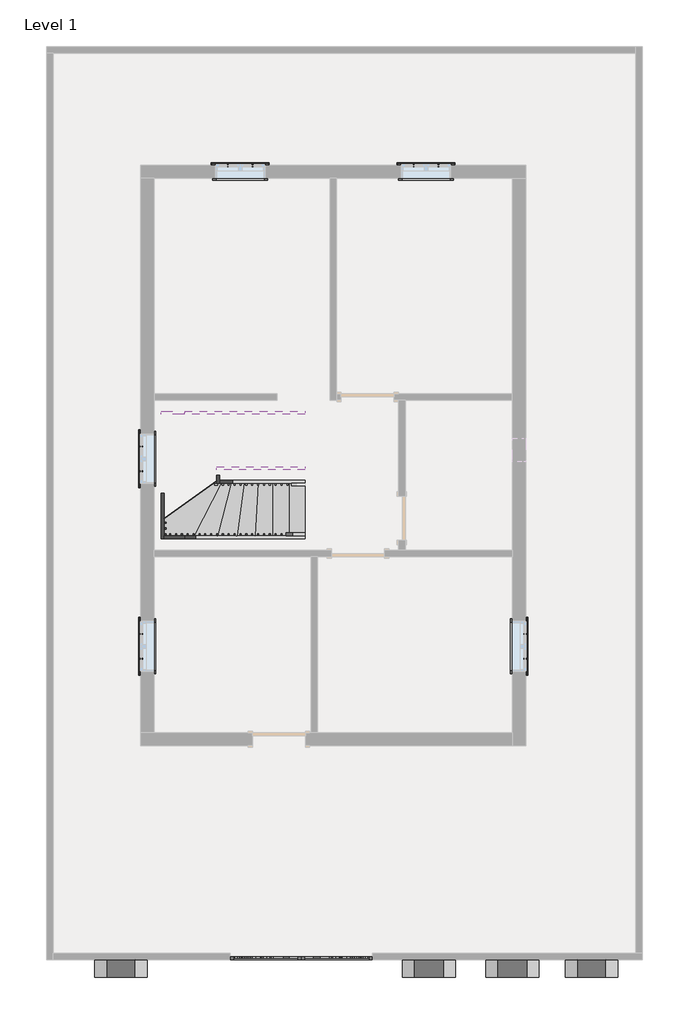
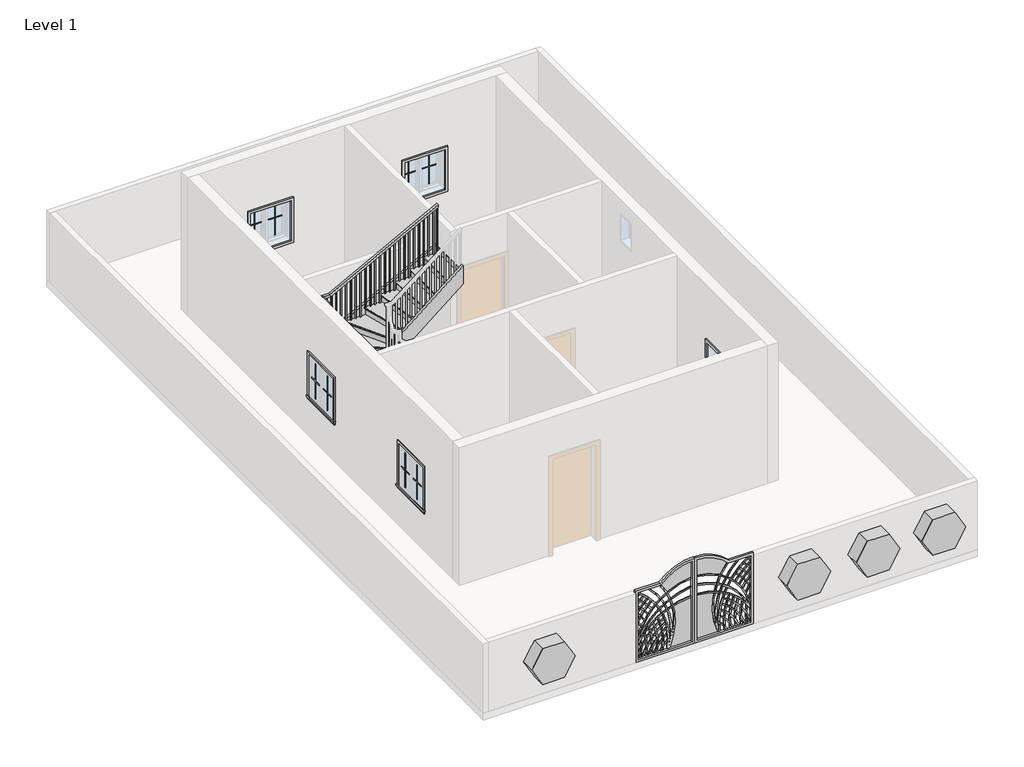
# One storey, part 2 of 2: 22 proxies, 8 members, 1 railing, 1 stair flight.
"""IFC4 building model written with IfcOpenShell, lengths in millimetres."""

from ifc_helpers import new_model, si_unit, frame, origin, place, context, project, spatial, polyline, outline, extrude, faceted_brep, transform, mapped, element, save
from components import generic_models_6bc30956, generic_models_2_generic_models_2_a86c904f, muntin_pattern_2x2_muntin_pattern_2x2_b3fe6957, muntin_pattern_2x2_muntin_pattern_2x2_3e0ecaf2, trim_window_exterior_flat_with_sill_41619996, trim_window_interior_flat_picture_frame_51c85655, stair_flight_5a9f065b

model = new_model("IFC4")

# Units and contexts
model_context = context("Model", 3, world=origin())
ifc_project = project(units=[si_unit("LENGTHUNIT", "METRE", prefix="MILLI")], contexts=[model_context])

# Site, building, storey
site = spatial("IfcSite", under=ifc_project)
building = spatial("IfcBuilding", under=site)
storey = spatial("IfcBuildingStorey", under=building, Name="Level 1", Elevation=0.0)

# Proxies
placement = place(None, origin())
generic_models_shape = generic_models_6bc30956(model_context)
element("IfcBuildingElementProxy", 1, Name="Generic Models", at=placement, inside=storey, context=model_context, shape_type="MappedRepresentation", body=[
    mapped(generic_models_shape, transform((-1831.5949167, -8550.141091, 0.0), x_axis=(1.0, 0.0, 0.0), y_axis=(0.0, 1.0, 0.0), z_axis=(0.0, 0.0, 1.0))),
])
generic_models_2_generic_models_2_shape = generic_models_2_generic_models_2_a86c904f(model_context)
element("IfcBuildingElementProxy", 2, Name="Generic Models 2 : Generic Models 2", ObjectType="Generic Models 2 : Generic Models 2", at=placement, inside=storey, context=model_context, shape_type="MappedRepresentation", body=[
    mapped(generic_models_2_generic_models_2_shape, transform((0.0, 0.0, 0.0), x_axis=(1.0, 0.0, 0.0), y_axis=(0.0, 1.0, 0.0), z_axis=(0.0, 0.0, 1.0))),
])
muntin_pattern_2x2_muntin_pattern_2x2_shape = muntin_pattern_2x2_muntin_pattern_2x2_b3fe6957(model_context)
element("IfcBuildingElementProxy", 3, Name="Muntin Pattern_2x2 : Muntin Pattern_2x2", ObjectType="Muntin Pattern_2x2 : Muntin Pattern_2x2", at=placement, inside=storey, context=model_context, shape_type="MappedRepresentation", body=[
    mapped(muntin_pattern_2x2_muntin_pattern_2x2_shape, transform((-3096.8324167, 5150.2179147, 984.25), x_axis=(1.0, 0.0, 0.0), y_axis=(0.0, 1.0, 0.0), z_axis=(0.0, 0.0, 1.0))),
])
element("IfcBuildingElementProxy", 4, Name="Muntin Pattern_2x2 : Muntin Pattern_2x2", ObjectType="Muntin Pattern_2x2 : Muntin Pattern_2x2", at=placement, inside=storey, context=model_context, shape_type="MappedRepresentation", body=[
    mapped(muntin_pattern_2x2_muntin_pattern_2x2_shape, transform((122.6175833, 5150.2179147, 984.25), x_axis=(1.0, 0.0, 0.0), y_axis=(0.0, 1.0, 0.0), z_axis=(0.0, 0.0, 1.0))),
])
element("IfcBuildingElementProxy", 5, Name="Muntin Pattern_2x2 : Muntin Pattern_2x2", ObjectType="Muntin Pattern_2x2 : Muntin Pattern_2x2", at=placement, inside=storey, context=model_context, shape_type="MappedRepresentation", body=[
    mapped(muntin_pattern_2x2_muntin_pattern_2x2_shape, transform((-4597.0199167, -3388.9445853, 984.25), x_axis=(0.0, 1.0, 0.0), y_axis=(-1.0, 0.0, 0.0), z_axis=(0.0, 0.0, 1.0))),
])
element("IfcBuildingElementProxy", 6, Name="Muntin Pattern_2x2 : Muntin Pattern_2x2", ObjectType="Muntin Pattern_2x2 : Muntin Pattern_2x2", at=placement, inside=storey, context=model_context, shape_type="MappedRepresentation", body=[
    mapped(muntin_pattern_2x2_muntin_pattern_2x2_shape, transform((2051.4300833, -2960.3195853, 984.25), x_axis=(0.0, -1.0, 0.0), y_axis=(1.0, 0.0, 0.0), z_axis=(0.0, 0.0, 1.0))),
])
element("IfcBuildingElementProxy", 7, Name="Muntin Pattern_2x2 : Muntin Pattern_2x2", ObjectType="Muntin Pattern_2x2 : Muntin Pattern_2x2", at=placement, inside=storey, context=model_context, shape_type="MappedRepresentation", body=[
    mapped(muntin_pattern_2x2_muntin_pattern_2x2_shape, transform((-4597.0199167, -140.9195853, 984.25), x_axis=(0.0, 1.0, 0.0), y_axis=(-1.0, 0.0, 0.0), z_axis=(0.0, 0.0, 1.0))),
])
muntin_pattern_2x2_muntin_pattern_2x2_2_shape = muntin_pattern_2x2_muntin_pattern_2x2_3e0ecaf2(model_context)
element("IfcBuildingElementProxy", 8, Name="Muntin Pattern_2x2 : Muntin Pattern_2x2", ObjectType="Muntin Pattern_2x2 : Muntin Pattern_2x2", at=placement, inside=storey, context=model_context, shape_type="MappedRepresentation", body=[
    mapped(muntin_pattern_2x2_muntin_pattern_2x2_2_shape, transform((-2668.2074167, 5150.2179147, 984.25), x_axis=(-1.0, 0.0, 0.0), y_axis=(0.0, -1.0, 0.0), z_axis=(0.0, 0.0, 1.0))),
])
element("IfcBuildingElementProxy", 9, Name="Muntin Pattern_2x2 : Muntin Pattern_2x2", ObjectType="Muntin Pattern_2x2 : Muntin Pattern_2x2", at=placement, inside=storey, context=model_context, shape_type="MappedRepresentation", body=[
    mapped(muntin_pattern_2x2_muntin_pattern_2x2_2_shape, transform((551.2425833, 5150.2179147, 984.25), x_axis=(-1.0, 0.0, 0.0), y_axis=(0.0, -1.0, 0.0), z_axis=(0.0, 0.0, 1.0))),
])
element("IfcBuildingElementProxy", 10, Name="Muntin Pattern_2x2 : Muntin Pattern_2x2", ObjectType="Muntin Pattern_2x2 : Muntin Pattern_2x2", at=placement, inside=storey, context=model_context, shape_type="MappedRepresentation", body=[
    mapped(muntin_pattern_2x2_muntin_pattern_2x2_2_shape, transform((-4597.0199167, -2960.3195853, 984.25), x_axis=(0.0, -1.0, 0.0), y_axis=(1.0, 0.0, 0.0), z_axis=(0.0, 0.0, 1.0))),
])
element("IfcBuildingElementProxy", 11, Name="Muntin Pattern_2x2 : Muntin Pattern_2x2", ObjectType="Muntin Pattern_2x2 : Muntin Pattern_2x2", at=placement, inside=storey, context=model_context, shape_type="MappedRepresentation", body=[
    mapped(muntin_pattern_2x2_muntin_pattern_2x2_2_shape, transform((2051.4300833, -3388.9445853, 984.25), x_axis=(0.0, 1.0, 0.0), y_axis=(-1.0, 0.0, 0.0), z_axis=(0.0, 0.0, 1.0))),
])
element("IfcBuildingElementProxy", 12, Name="Muntin Pattern_2x2 : Muntin Pattern_2x2", ObjectType="Muntin Pattern_2x2 : Muntin Pattern_2x2", at=placement, inside=storey, context=model_context, shape_type="MappedRepresentation", body=[
    mapped(muntin_pattern_2x2_muntin_pattern_2x2_2_shape, transform((-4597.0199167, 287.7054147, 984.25), x_axis=(0.0, -1.0, 0.0), y_axis=(1.0, 0.0, 0.0), z_axis=(0.0, 0.0, 1.0))),
])
trim_window_exterior_flat_with_sill_shape = trim_window_exterior_flat_with_sill_41619996(model_context)
element("IfcBuildingElementProxy", 13, Name="Trim-Window-Exterior-Flat : with Sill", ObjectType="Trim-Window-Exterior-Flat : with Sill", at=placement, inside=storey, context=model_context, shape_type="MappedRepresentation", body=[
    mapped(trim_window_exterior_flat_with_sill_shape, transform((-2882.5199167, 5159.7429147, 1828.8), x_axis=(-1.0, 0.0, 0.0), y_axis=(0.0, 0.0, 1.0), z_axis=(0.0, 1.0, 0.0))),
])
element("IfcBuildingElementProxy", 14, Name="Trim-Window-Exterior-Flat : with Sill", ObjectType="Trim-Window-Exterior-Flat : with Sill", at=placement, inside=storey, context=model_context, shape_type="MappedRepresentation", body=[
    mapped(trim_window_exterior_flat_with_sill_shape, transform((336.9300833, 5159.7429147, 1828.8), x_axis=(-1.0, 0.0, 0.0), y_axis=(0.0, 0.0, 1.0), z_axis=(0.0, 1.0, 0.0))),
])
element("IfcBuildingElementProxy", 15, Name="Trim-Window-Exterior-Flat : with Sill", ObjectType="Trim-Window-Exterior-Flat : with Sill", at=placement, inside=storey, context=model_context, shape_type="MappedRepresentation", body=[
    mapped(trim_window_exterior_flat_with_sill_shape, transform((-4606.5449167, -3174.6320853, 1828.8), x_axis=(0.0, -1.0, 0.0), y_axis=(0.0, 0.0, 1.0), z_axis=(-1.0, 0.0, 0.0))),
])
element("IfcBuildingElementProxy", 16, Name="Trim-Window-Exterior-Flat : with Sill", ObjectType="Trim-Window-Exterior-Flat : with Sill", at=placement, inside=storey, context=model_context, shape_type="MappedRepresentation", body=[
    mapped(trim_window_exterior_flat_with_sill_shape, transform((2060.9550833, -3174.6320853, 1828.8), x_axis=(0.0, 1.0, 0.0), y_axis=(0.0, 0.0, 1.0), z_axis=(1.0, 0.0, 0.0))),
])
element("IfcBuildingElementProxy", 17, Name="Trim-Window-Exterior-Flat : with Sill", ObjectType="Trim-Window-Exterior-Flat : with Sill", at=placement, inside=storey, context=model_context, shape_type="MappedRepresentation", body=[
    mapped(trim_window_exterior_flat_with_sill_shape, transform((-4606.5449167, 73.3929147, 1828.8), x_axis=(0.0, -1.0, 0.0), y_axis=(0.0, 0.0, 1.0), z_axis=(-1.0, 0.0, 0.0))),
])
trim_window_interior_flat_picture_frame_shape = trim_window_interior_flat_picture_frame_51c85655(model_context)
element("IfcBuildingElementProxy", 18, Name="Trim-Window-Interior-Flat : Picture Frame", ObjectType="Trim-Window-Interior-Flat : Picture Frame", at=placement, inside=storey, context=model_context, shape_type="MappedRepresentation", body=[
    mapped(trim_window_interior_flat_picture_frame_shape, transform((-2882.5199167, 4931.1429147, 1828.8), x_axis=(1.0, 0.0, 0.0), y_axis=(0.0, 0.0, 1.0), z_axis=(0.0, -1.0, 0.0))),
])
element("IfcBuildingElementProxy", 19, Name="Trim-Window-Interior-Flat : Picture Frame", ObjectType="Trim-Window-Interior-Flat : Picture Frame", at=placement, inside=storey, context=model_context, shape_type="MappedRepresentation", body=[
    mapped(trim_window_interior_flat_picture_frame_shape, transform((336.9300833, 4931.1429147, 1828.8), x_axis=(1.0, 0.0, 0.0), y_axis=(0.0, 0.0, 1.0), z_axis=(0.0, -1.0, 0.0))),
])
element("IfcBuildingElementProxy", 20, Name="Trim-Window-Interior-Flat : Picture Frame", ObjectType="Trim-Window-Interior-Flat : Picture Frame", at=placement, inside=storey, context=model_context, shape_type="MappedRepresentation", body=[
    mapped(trim_window_interior_flat_picture_frame_shape, transform((-4377.9449167, -3174.6320853, 1828.8), x_axis=(0.0, 1.0, 0.0), y_axis=(0.0, 0.0, 1.0), z_axis=(1.0, 0.0, 0.0))),
])
element("IfcBuildingElementProxy", 21, Name="Trim-Window-Interior-Flat : Picture Frame", ObjectType="Trim-Window-Interior-Flat : Picture Frame", at=placement, inside=storey, context=model_context, shape_type="MappedRepresentation", body=[
    mapped(trim_window_interior_flat_picture_frame_shape, transform((1832.3550833, -3174.6320853, 1828.8), x_axis=(0.0, -1.0, 0.0), y_axis=(0.0, 0.0, 1.0), z_axis=(-1.0, 0.0, 0.0))),
])
element("IfcBuildingElementProxy", 22, Name="Trim-Window-Interior-Flat : Picture Frame", ObjectType="Trim-Window-Interior-Flat : Picture Frame", at=placement, inside=storey, context=model_context, shape_type="MappedRepresentation", body=[
    mapped(trim_window_interior_flat_picture_frame_shape, transform((-4377.9449167, 73.3929147, 1828.8), x_axis=(0.0, 1.0, 0.0), y_axis=(0.0, 0.0, 1.0), z_axis=(1.0, 0.0, 0.0))),
])

# Members
element("IfcMember", 23, ObjectType="Stringer - 2\" Width", at=placement, inside=storey, context=model_context, shape_type="SweptSolid", body=[
    extrude(outline(polyline([(0.0, -1761.7449167), (229.639954, -1761.7449167), (1305.3956453, -3849.1621084), (962.500629, -3849.1621084), (0.0, -1981.5072342), (0.0, -1761.7449167)])), frame((0.0, -1310.9070853, 0.0), z_axis=(0.0, 1.0, 0.0), x_axis=(0.0, 0.0, 1.0)), (0.0, 0.0, 1.0), 50.8),
])
element("IfcMember", 24, ObjectType="Stringer - 2\" Width", at=placement, inside=storey, context=model_context, shape_type="SweptSolid", body=[
    extrude(outline(polyline([(-3849.1621084, -1260.1070853), (-3849.1621084, -1310.9070853), (-4203.8766085, -1310.9070853), (-4203.8766085, -1260.1070853), (-3849.1621084, -1260.1070853)])), frame((0.0, 0.0, 962.500629), z_axis=(0.0, 0.0, 1.0), x_axis=(1.0, 0.0, 0.0)), (0.0, 0.0, 1.0), 342.8950162),
])
element("IfcMember", 25, ObjectType="Stringer - 2\" Width", at=placement, inside=storey, context=model_context, shape_type="SweptSolid", body=[
    extrude(outline(polyline([(-1310.9070853, 1000.5956453), (-1310.9070853, 1289.0952212), (811.1127974, 1969.9972697), (848.0929147, 1969.9972697), (848.0929147, 1638.9682298), (-1141.3846024, 1000.5956453), (-1310.9070853, 1000.5956453)])), frame((-4254.6766085, 0.0, 0.0), z_axis=(1.0, 0.0, 0.0), x_axis=(0.0, 1.0, 0.0)), (0.0, 0.0, 1.0), 50.8),
])
element("IfcMember", 26, ObjectType="Stringer - 2\" Width", at=placement, inside=storey, context=model_context, shape_type="SweptSolid", body=[
    extrude(outline(polyline([(-4254.6766085, 848.0929147), (-4254.6766085, 898.8929147), (-3849.1621084, 898.8929147), (-3849.1621084, 848.0929147), (-4254.6766085, 848.0929147)])), frame((0.0, 0.0, 1649.8904473), z_axis=(0.0, 0.0, 1.0), x_axis=(1.0, 0.0, 0.0)), (0.0, 0.0, 1.0), 320.1068224),
])
element("IfcMember", 27, ObjectType="Stringer - 2\" Width", at=placement, inside=storey, context=model_context, shape_type="SweptSolid", body=[
    extrude(outline(polyline([(1969.9972697, -3849.1621084), (1649.8904473, -3849.1621084), (2725.6461385, -1761.7449167), (3045.7529609, -1761.7449167), (1969.9972697, -3849.1621084)])), frame((0.0, 848.0929147, 0.0), z_axis=(0.0, 1.0, 0.0), x_axis=(0.0, 0.0, 1.0)), (0.0, 0.0, 1.0), 50.8),
])
element("IfcMember", 28, ObjectType="Stringer - 2\" Width", at=placement, inside=storey, context=model_context, shape_type="SweptSolid", body=[
    extrude(outline(polyline([(0.0, -1761.7449167), (176.1764461, -1761.7449167), (1380.418648, -3238.6766085), (987.1410923, -3238.6766085), (0.0, -2028.0065612), (0.0, -1761.7449167)])), frame((0.0, -345.7070853, 0.0), z_axis=(0.0, 1.0, 0.0), x_axis=(0.0, 0.0, 1.0)), (0.0, 0.0, 1.0), 50.8),
])
element("IfcMember", 29, ObjectType="Stringer - 2\" Width", at=placement, inside=storey, context=model_context, shape_type="SweptSolid", body=[
    extrude(outline(polyline([(-345.7070853, 1028.5617647), (-345.7070853, 1573.2682978), (-139.0699679, 1926.1409689), (-117.1070853, 1926.1409689), (-117.1070853, 1360.465107), (-311.464868, 1028.5617647), (-345.7070853, 1028.5617647)])), frame((-3289.4766085, 0.0, 0.0), z_axis=(1.0, 0.0, 0.0), x_axis=(0.0, 1.0, 0.0)), (0.0, 0.0, 1.0), 50.8),
])
element("IfcMember", 30, ObjectType="Stringer - 2\" Width", at=placement, inside=storey, context=model_context, shape_type="SweptSolid", body=[
    extrude(outline(polyline([(1926.1409689, -3289.4766085), (1532.8634131, -3289.4766085), (2778.5262875, -1761.7449167), (3171.8038432, -1761.7449167), (1926.1409689, -3289.4766085)])), frame((0.0, -117.1070853, 0.0), z_axis=(0.0, 1.0, 0.0), x_axis=(0.0, 0.0, 1.0)), (0.0, 0.0, 1.0), 50.8),
])

# Railing
element("IfcRailing", 31, ObjectType="Handrail - Rectangular", at=placement, inside=storey, context=model_context, shape_type="SolidModel", body=[
    faceted_brep([(-1761.7449167, -1260.1070853, 1083.7333333), (-1761.7449167, -1260.1070853, 1026.2742652), (-1761.7449167, -1209.3070853, 1026.2742652), (-1761.7449167, -1209.3070853, 1083.7333333), (-4019.4699787, -1260.1070853, 2277.0239201), (-4032.0690433, -1260.1070853, 2226.2239201), (-4032.0690433, -1209.3070853, 2226.2239201), (-4019.4699787, -1209.3070853, 2277.0239201), (-4203.8766085, -1260.1070853, 2277.0239201), (-4203.8766085, -1260.1070853, 2226.2239201), (-4153.0766085, -1209.3070853, 2226.2239201), (-4153.0766085, -1209.3070853, 2277.0239201), (-4203.8766085, -972.7952032, 2277.0239201), (-4203.8766085, -964.8446271, 2226.2239201), (-4153.0766085, -964.8446271, 2226.2239201), (-4153.0766085, -972.7952032, 2277.0239201), (-4203.8766085, 560.7810325, 2769.1094132), (-4203.8766085, 568.7316087, 2718.3094132), (-4153.0766085, 568.7316087, 2718.3094132), (-4153.0766085, 560.7810325, 2769.1094132), (-4203.8766085, 848.0929147, 2769.1094132), (-4203.8766085, 848.0929147, 2718.3094132), (-4153.0766085, 797.2929147, 2718.3094132), (-4153.0766085, 797.2929147, 2769.1094132), (-4019.4699787, 848.0929147, 2769.1094132), (-4006.8709142, 848.0929147, 2718.3094132), (-4006.8709142, 797.2929147, 2718.3094132), (-4019.4699787, 797.2929147, 2769.1094132), (-1761.7449167, 848.0929147, 3962.4), (-1761.7449167, 797.2929147, 3962.4), (-1761.7449167, 797.2929147, 3904.9409318), (-1761.7449167, 848.0929147, 3904.9409318)], [[[0, 1, 2, 3]], [[1, 0, 4, 5]], [[2, 1, 5, 6]], [[3, 2, 6, 7]], [[0, 3, 7, 4]], [[5, 4, 8, 9]], [[6, 5, 9, 10]], [[7, 6, 10, 11]], [[4, 7, 11, 8]], [[9, 8, 12, 13]], [[10, 9, 13, 14]], [[11, 10, 14, 15]], [[8, 11, 15, 12]], [[13, 12, 16, 17]], [[14, 13, 17, 18]], [[15, 14, 18, 19]], [[12, 15, 19, 16]], [[17, 16, 20, 21]], [[18, 17, 21, 22]], [[19, 18, 22, 23]], [[16, 19, 23, 20]], [[21, 20, 24, 25]], [[22, 21, 25, 26]], [[23, 22, 26, 27]], [[20, 23, 27, 24]], [[28, 29, 30, 31]], [[25, 24, 28, 31]], [[26, 25, 31, 30]], [[27, 26, 30, 29]], [[24, 27, 29, 28]]]),
    extrude(outline(polyline([(3857.6597858, -1851.2016085), (2878.6666667, -1851.2016085), (2878.6666667, -1832.1516085), (3867.7284102, -1832.1516085), (3857.6597858, -1851.2016085)])), frame((0.0, 813.1679147, 0.0), z_axis=(0.0, 1.0, 0.0), x_axis=(0.0, 0.0, 1.0)), (0.0, 0.0, 1.0), 19.05),
    extrude(outline(polyline([(3803.9604556, -1952.8016085), (2878.6666667, -1952.8016085), (2878.6666667, -1933.7516085), (3814.02908, -1933.7516085), (3803.9604556, -1952.8016085)])), frame((0.0, 813.1679147, 0.0), z_axis=(0.0, 1.0, 0.0), x_axis=(0.0, 0.0, 1.0)), (0.0, 0.0, 1.0), 19.05),
    extrude(outline(polyline([(3750.2611254, -2054.4016085), (2709.3333333, -2054.4016085), (2709.3333333, -2035.3516085), (3760.3297498, -2035.3516085), (3750.2611254, -2054.4016085)])), frame((0.0, 813.1679147, 0.0), z_axis=(0.0, 1.0, 0.0), x_axis=(0.0, 0.0, 1.0)), (0.0, 0.0, 1.0), 19.05),
    extrude(outline(polyline([(3696.5617952, -2156.0016085), (2709.3333333, -2156.0016085), (2709.3333333, -2136.9516085), (3706.6304196, -2136.9516085), (3696.5617952, -2156.0016085)])), frame((0.0, 813.1679147, 0.0), z_axis=(0.0, 1.0, 0.0), x_axis=(0.0, 0.0, 1.0)), (0.0, 0.0, 1.0), 19.05),
    extrude(outline(polyline([(3642.862465, -2257.6016085), (2709.3333333, -2257.6016085), (2709.3333333, -2238.5516085), (3652.9310894, -2238.5516085), (3642.862465, -2257.6016085)])), frame((0.0, 813.1679147, 0.0), z_axis=(0.0, 1.0, 0.0), x_axis=(0.0, 0.0, 1.0)), (0.0, 0.0, 1.0), 19.05),
    extrude(outline(polyline([(3589.1631348, -2359.2016085), (2540.0, -2359.2016085), (2540.0, -2340.1516085), (3599.2317592, -2340.1516085), (3589.1631348, -2359.2016085)])), frame((0.0, 813.1679147, 0.0), z_axis=(0.0, 1.0, 0.0), x_axis=(0.0, 0.0, 1.0)), (0.0, 0.0, 1.0), 19.05),
    extrude(outline(polyline([(3535.4638046, -2460.8016085), (2540.0, -2460.8016085), (2540.0, -2441.7516085), (3545.532429, -2441.7516085), (3535.4638046, -2460.8016085)])), frame((0.0, 813.1679147, 0.0), z_axis=(0.0, 1.0, 0.0), x_axis=(0.0, 0.0, 1.0)), (0.0, 0.0, 1.0), 19.05),
    extrude(outline(polyline([(3481.7644744, -2562.4016085), (2540.0, -2562.4016085), (2540.0, -2543.3516085), (3491.8330988, -2543.3516085), (3481.7644744, -2562.4016085)])), frame((0.0, 813.1679147, 0.0), z_axis=(0.0, 1.0, 0.0), x_axis=(0.0, 0.0, 1.0)), (0.0, 0.0, 1.0), 19.05),
    extrude(outline(polyline([(3428.0651442, -2664.0016085), (2370.6666667, -2664.0016085), (2370.6666667, -2644.9516085), (3438.1337686, -2644.9516085), (3428.0651442, -2664.0016085)])), frame((0.0, 813.1679147, 0.0), z_axis=(0.0, 1.0, 0.0), x_axis=(0.0, 0.0, 1.0)), (0.0, 0.0, 1.0), 19.05),
    extrude(outline(polyline([(3374.365814, -2765.6016085), (2370.6666667, -2765.6016085), (2370.6666667, -2746.5516085), (3384.4344384, -2746.5516085), (3374.365814, -2765.6016085)])), frame((0.0, 813.1679147, 0.0), z_axis=(0.0, 1.0, 0.0), x_axis=(0.0, 0.0, 1.0)), (0.0, 0.0, 1.0), 19.05),
    extrude(outline(polyline([(3320.6664838, -2867.2016085), (2370.6666667, -2867.2016085), (2370.6666667, -2848.1516085), (3330.7351082, -2848.1516085), (3320.6664838, -2867.2016085)])), frame((0.0, 813.1679147, 0.0), z_axis=(0.0, 1.0, 0.0), x_axis=(0.0, 0.0, 1.0)), (0.0, 0.0, 1.0), 19.05),
    extrude(outline(polyline([(3266.9671536, -2968.8016085), (2201.3333333, -2968.8016085), (2201.3333333, -2949.7516085), (3277.035778, -2949.7516085), (3266.9671536, -2968.8016085)])), frame((0.0, 813.1679147, 0.0), z_axis=(0.0, 1.0, 0.0), x_axis=(0.0, 0.0, 1.0)), (0.0, 0.0, 1.0), 19.05),
    extrude(outline(polyline([(3213.2678234, -3070.4016085), (2201.3333333, -3070.4016085), (2201.3333333, -3051.3516085), (3223.3364478, -3051.3516085), (3213.2678234, -3070.4016085)])), frame((0.0, 813.1679147, 0.0), z_axis=(0.0, 1.0, 0.0), x_axis=(0.0, 0.0, 1.0)), (0.0, 0.0, 1.0), 19.05),
    extrude(outline(polyline([(3159.5684932, -3172.0016085), (2201.3333333, -3172.0016085), (2201.3333333, -3152.9516085), (3169.6371176, -3152.9516085), (3159.5684932, -3172.0016085)])), frame((0.0, 813.1679147, 0.0), z_axis=(0.0, 1.0, 0.0), x_axis=(0.0, 0.0, 1.0)), (0.0, 0.0, 1.0), 19.05),
    extrude(outline(polyline([(3105.869163, -3273.6016085), (2201.3333333, -3273.6016085), (2201.3333333, -3254.5516085), (3115.9377874, -3254.5516085), (3105.869163, -3273.6016085)])), frame((0.0, 813.1679147, 0.0), z_axis=(0.0, 1.0, 0.0), x_axis=(0.0, 0.0, 1.0)), (0.0, 0.0, 1.0), 19.05),
    extrude(outline(polyline([(3052.1698328, -3375.2016085), (2032.0, -3375.2016085), (2032.0, -3356.1516085), (3062.2384572, -3356.1516085), (3052.1698328, -3375.2016085)])), frame((0.0, 813.1679147, 0.0), z_axis=(0.0, 1.0, 0.0), x_axis=(0.0, 0.0, 1.0)), (0.0, 0.0, 1.0), 19.05),
    extrude(outline(polyline([(2998.4705026, -3476.8016085), (2032.0, -3476.8016085), (2032.0, -3457.7516085), (3008.539127, -3457.7516085), (2998.4705026, -3476.8016085)])), frame((0.0, 813.1679147, 0.0), z_axis=(0.0, 1.0, 0.0), x_axis=(0.0, 0.0, 1.0)), (0.0, 0.0, 1.0), 19.05),
    extrude(outline(polyline([(2944.7711724, -3578.4016085), (2032.0, -3578.4016085), (2032.0, -3559.3516085), (2954.8397968, -3559.3516085), (2944.7711724, -3578.4016085)])), frame((0.0, 813.1679147, 0.0), z_axis=(0.0, 1.0, 0.0), x_axis=(0.0, 0.0, 1.0)), (0.0, 0.0, 1.0), 19.05),
    extrude(outline(polyline([(2891.0718422, -3680.0016085), (2032.0, -3680.0016085), (2032.0, -3660.9516085), (2901.1404666, -3660.9516085), (2891.0718422, -3680.0016085)])), frame((0.0, 813.1679147, 0.0), z_axis=(0.0, 1.0, 0.0), x_axis=(0.0, 0.0, 1.0)), (0.0, 0.0, 1.0), 19.05),
    extrude(outline(polyline([(2837.372512, -3781.6016085), (1862.6666667, -3781.6016085), (1862.6666667, -3762.5516085), (2847.4411364, -3762.5516085), (2837.372512, -3781.6016085)])), frame((0.0, 813.1679147, 0.0), z_axis=(0.0, 1.0, 0.0), x_axis=(0.0, 0.0, 1.0)), (0.0, 0.0, 1.0), 19.05),
    extrude(outline(polyline([(2783.6731818, -3883.2016085), (1862.6666667, -3883.2016085), (1862.6666667, -3864.1516085), (2793.7418062, -3864.1516085), (2783.6731818, -3883.2016085)])), frame((0.0, 813.1679147, 0.0), z_axis=(0.0, 1.0, 0.0), x_axis=(0.0, 0.0, 1.0)), (0.0, 0.0, 1.0), 19.05),
    extrude(outline(polyline([(2729.9738516, -3984.8016085), (1862.6666667, -3984.8016085), (1862.6666667, -3965.7516085), (2740.042476, -3965.7516085), (2729.9738516, -3984.8016085)])), frame((0.0, 813.1679147, 0.0), z_axis=(0.0, 1.0, 0.0), x_axis=(0.0, 0.0, 1.0)), (0.0, 0.0, 1.0), 19.05),
    extrude(outline(polyline([(-4086.4016085, 832.2179147), (-4067.3516085, 832.2179147), (-4067.3516085, 813.1679147), (-4086.4016085, 813.1679147), (-4086.4016085, 832.2179147)])), frame((0.0, 0.0, 1862.6666667), z_axis=(0.0, 0.0, 1.0), x_axis=(1.0, 0.0, 0.0)), (0.0, 0.0, 1.0), 855.6427466),
    extrude(outline(polyline([(-4188.0016085, 787.7679147), (-4188.0016085, 806.8179147), (-4168.9516085, 806.8179147), (-4168.9516085, 787.7679147), (-4188.0016085, 787.7679147)])), frame((0.0, 0.0, 1862.6666667), z_axis=(0.0, 0.0, 1.0), x_axis=(1.0, 0.0, 0.0)), (0.0, 0.0, 1.0), 855.6427466),
    extrude(outline(polyline([(-4188.0016085, 686.1679147), (-4188.0016085, 705.2179147), (-4168.9516085, 705.2179147), (-4168.9516085, 686.1679147), (-4188.0016085, 686.1679147)])), frame((0.0, 0.0, 1862.6666667), z_axis=(0.0, 0.0, 1.0), x_axis=(1.0, 0.0, 0.0)), (0.0, 0.0, 1.0), 855.6427466),
    extrude(outline(polyline([(-4188.0016085, 584.5679147), (-4188.0016085, 603.6179147), (-4168.9516085, 603.6179147), (-4168.9516085, 584.5679147), (-4188.0016085, 584.5679147)])), frame((0.0, 0.0, 1862.6666667), z_axis=(0.0, 0.0, 1.0), x_axis=(1.0, 0.0, 0.0)), (0.0, 0.0, 1.0), 855.6427466),
    extrude(outline(polyline([(502.0179147, 2696.9026907), (502.0179147, 1693.3333333), (482.9679147, 1693.3333333), (482.9679147, 2690.7900316), (502.0179147, 2696.9026907)])), frame((-4188.0016085, 0.0, 0.0), z_axis=(1.0, 0.0, 0.0), x_axis=(0.0, 1.0, 0.0)), (0.0, 0.0, 1.0), 19.05),
    extrude(outline(polyline([(400.4179147, 2664.3018425), (400.4179147, 1693.3333333), (381.3679147, 1693.3333333), (381.3679147, 2658.1891834), (400.4179147, 2664.3018425)])), frame((-4188.0016085, 0.0, 0.0), z_axis=(1.0, 0.0, 0.0), x_axis=(0.0, 1.0, 0.0)), (0.0, 0.0, 1.0), 19.05),
    extrude(outline(polyline([(298.8179147, 2631.7009942), (298.8179147, 1693.3333333), (279.7679147, 1693.3333333), (279.7679147, 2625.5883352), (298.8179147, 2631.7009942)])), frame((-4188.0016085, 0.0, 0.0), z_axis=(1.0, 0.0, 0.0), x_axis=(0.0, 1.0, 0.0)), (0.0, 0.0, 1.0), 19.05),
    extrude(outline(polyline([(197.2179147, 2599.100146), (197.2179147, 1693.3333333), (178.1679147, 1693.3333333), (178.1679147, 2592.987487), (197.2179147, 2599.100146)])), frame((-4188.0016085, 0.0, 0.0), z_axis=(1.0, 0.0, 0.0), x_axis=(0.0, 1.0, 0.0)), (0.0, 0.0, 1.0), 19.05),
    extrude(outline(polyline([(95.6179147, 2566.4992978), (95.6179147, 1693.3333333), (76.5679147, 1693.3333333), (76.5679147, 2560.3866387), (95.6179147, 2566.4992978)])), frame((-4188.0016085, 0.0, 0.0), z_axis=(1.0, 0.0, 0.0), x_axis=(0.0, 1.0, 0.0)), (0.0, 0.0, 1.0), 19.05),
    extrude(outline(polyline([(-5.9820853, 2533.8984495), (-5.9820853, 1524.0), (-25.0320853, 1524.0), (-25.0320853, 2527.7857905), (-5.9820853, 2533.8984495)])), frame((-4188.0016085, 0.0, 0.0), z_axis=(1.0, 0.0, 0.0), x_axis=(0.0, 1.0, 0.0)), (0.0, 0.0, 1.0), 19.05),
    extrude(outline(polyline([(-107.5820853, 2501.2976013), (-107.5820853, 1524.0), (-126.6320853, 1524.0), (-126.6320853, 2495.1849423), (-107.5820853, 2501.2976013)])), frame((-4188.0016085, 0.0, 0.0), z_axis=(1.0, 0.0, 0.0), x_axis=(0.0, 1.0, 0.0)), (0.0, 0.0, 1.0), 19.05),
    extrude(outline(polyline([(-209.1820853, 2468.6967531), (-209.1820853, 1524.0), (-228.2320853, 1524.0), (-228.2320853, 2462.5840941), (-209.1820853, 2468.6967531)])), frame((-4188.0016085, 0.0, 0.0), z_axis=(1.0, 0.0, 0.0), x_axis=(0.0, 1.0, 0.0)), (0.0, 0.0, 1.0), 19.05),
    extrude(outline(polyline([(-310.7820853, 2436.0959049), (-310.7820853, 1524.0), (-329.8320853, 1524.0), (-329.8320853, 2429.9832458), (-310.7820853, 2436.0959049)])), frame((-4188.0016085, 0.0, 0.0), z_axis=(1.0, 0.0, 0.0), x_axis=(0.0, 1.0, 0.0)), (0.0, 0.0, 1.0), 19.05),
    extrude(outline(polyline([(-412.3820853, 2403.4950566), (-412.3820853, 1524.0), (-431.4320853, 1524.0), (-431.4320853, 2397.3823976), (-412.3820853, 2403.4950566)])), frame((-4188.0016085, 0.0, 0.0), z_axis=(1.0, 0.0, 0.0), x_axis=(0.0, 1.0, 0.0)), (0.0, 0.0, 1.0), 19.05),
    extrude(outline(polyline([(-513.9820853, 2370.8942084), (-513.9820853, 1354.6666667), (-533.0320853, 1354.6666667), (-533.0320853, 2364.7815494), (-513.9820853, 2370.8942084)])), frame((-4188.0016085, 0.0, 0.0), z_axis=(1.0, 0.0, 0.0), x_axis=(0.0, 1.0, 0.0)), (0.0, 0.0, 1.0), 19.05),
    extrude(outline(polyline([(-615.5820853, 2338.2933602), (-615.5820853, 1354.6666667), (-634.6320853, 1354.6666667), (-634.6320853, 2332.1807011), (-615.5820853, 2338.2933602)])), frame((-4188.0016085, 0.0, 0.0), z_axis=(1.0, 0.0, 0.0), x_axis=(0.0, 1.0, 0.0)), (0.0, 0.0, 1.0), 19.05),
    extrude(outline(polyline([(-717.1820853, 2305.692512), (-717.1820853, 1354.6666667), (-736.2320853, 1354.6666667), (-736.2320853, 2299.5798529), (-717.1820853, 2305.692512)])), frame((-4188.0016085, 0.0, 0.0), z_axis=(1.0, 0.0, 0.0), x_axis=(0.0, 1.0, 0.0)), (0.0, 0.0, 1.0), 19.05),
    extrude(outline(polyline([(-818.7820853, 2273.0916637), (-818.7820853, 1354.6666667), (-837.8320853, 1354.6666667), (-837.8320853, 2266.9790047), (-818.7820853, 2273.0916637)])), frame((-4188.0016085, 0.0, 0.0), z_axis=(1.0, 0.0, 0.0), x_axis=(0.0, 1.0, 0.0)), (0.0, 0.0, 1.0), 19.05),
    extrude(outline(polyline([(-920.3820853, 2240.4908155), (-920.3820853, 1354.6666667), (-939.4320853, 1354.6666667), (-939.4320853, 2234.3781565), (-920.3820853, 2240.4908155)])), frame((-4188.0016085, 0.0, 0.0), z_axis=(1.0, 0.0, 0.0), x_axis=(0.0, 1.0, 0.0)), (0.0, 0.0, 1.0), 19.05),
    extrude(outline(polyline([(-4188.0016085, -1041.0320853), (-4188.0016085, -1021.9820853), (-4168.9516085, -1021.9820853), (-4168.9516085, -1041.0320853), (-4188.0016085, -1041.0320853)])), frame((0.0, 0.0, 1185.3333333), z_axis=(0.0, 0.0, 1.0), x_axis=(1.0, 0.0, 0.0)), (0.0, 0.0, 1.0), 1040.8905868),
    extrude(outline(polyline([(-4188.0016085, -1142.6320853), (-4188.0016085, -1123.5820853), (-4168.9516085, -1123.5820853), (-4168.9516085, -1142.6320853), (-4188.0016085, -1142.6320853)])), frame((0.0, 0.0, 1185.3333333), z_axis=(0.0, 0.0, 1.0), x_axis=(1.0, 0.0, 0.0)), (0.0, 0.0, 1.0), 1040.8905868),
    extrude(outline(polyline([(-4089.0199167, -1244.2320853), (-4108.0699167, -1244.2320853), (-4108.0699167, -1225.1820853), (-4089.0199167, -1225.1820853), (-4089.0199167, -1244.2320853)])), frame((0.0, 0.0, 1185.3333333), z_axis=(0.0, 0.0, 1.0), x_axis=(1.0, 0.0, 0.0)), (0.0, 0.0, 1.0), 1040.8905868),
    extrude(outline(polyline([(2212.6938418, -4006.4699167), (1185.3333333, -4006.4699167), (1185.3333333, -3987.4199167), (2202.6252174, -3987.4199167), (2212.6938418, -4006.4699167)])), frame((0.0, -1244.2320853, 0.0), z_axis=(0.0, 1.0, 0.0), x_axis=(0.0, 0.0, 1.0)), (0.0, 0.0, 1.0), 19.05),
    extrude(outline(polyline([(2158.9945116, -3904.8699167), (1185.3333333, -3904.8699167), (1185.3333333, -3885.8199167), (2148.9258872, -3885.8199167), (2158.9945116, -3904.8699167)])), frame((0.0, -1244.2320853, 0.0), z_axis=(0.0, 1.0, 0.0), x_axis=(0.0, 0.0, 1.0)), (0.0, 0.0, 1.0), 19.05),
    extrude(outline(polyline([(2105.2951814, -3803.2699167), (1185.3333333, -3803.2699167), (1185.3333333, -3784.2199167), (2095.226557, -3784.2199167), (2105.2951814, -3803.2699167)])), frame((0.0, -1244.2320853, 0.0), z_axis=(0.0, 1.0, 0.0), x_axis=(0.0, 0.0, 1.0)), (0.0, 0.0, 1.0), 19.05),
    extrude(outline(polyline([(2051.5958512, -3701.6699167), (1185.3333333, -3701.6699167), (1185.3333333, -3682.6199167), (2041.5272268, -3682.6199167), (2051.5958512, -3701.6699167)])), frame((0.0, -1244.2320853, 0.0), z_axis=(0.0, 1.0, 0.0), x_axis=(0.0, 0.0, 1.0)), (0.0, 0.0, 1.0), 19.05),
    extrude(outline(polyline([(1997.896521, -3600.0699167), (1016.0, -3600.0699167), (1016.0, -3581.0199167), (1987.8278966, -3581.0199167), (1997.896521, -3600.0699167)])), frame((0.0, -1244.2320853, 0.0), z_axis=(0.0, 1.0, 0.0), x_axis=(0.0, 0.0, 1.0)), (0.0, 0.0, 1.0), 19.05),
    extrude(outline(polyline([(1944.1971908, -3498.4699167), (1016.0, -3498.4699167), (1016.0, -3479.4199167), (1934.1285664, -3479.4199167), (1944.1971908, -3498.4699167)])), frame((0.0, -1244.2320853, 0.0), z_axis=(0.0, 1.0, 0.0), x_axis=(0.0, 0.0, 1.0)), (0.0, 0.0, 1.0), 19.05),
    extrude(outline(polyline([(1890.4978606, -3396.8699167), (1016.0, -3396.8699167), (1016.0, -3377.8199167), (1880.4292362, -3377.8199167), (1890.4978606, -3396.8699167)])), frame((0.0, -1244.2320853, 0.0), z_axis=(0.0, 1.0, 0.0), x_axis=(0.0, 0.0, 1.0)), (0.0, 0.0, 1.0), 19.05),
    extrude(outline(polyline([(1836.7985304, -3295.2699167), (1016.0, -3295.2699167), (1016.0, -3276.2199167), (1826.729906, -3276.2199167), (1836.7985304, -3295.2699167)])), frame((0.0, -1244.2320853, 0.0), z_axis=(0.0, 1.0, 0.0), x_axis=(0.0, 0.0, 1.0)), (0.0, 0.0, 1.0), 19.05),
    extrude(outline(polyline([(1783.0992002, -3193.6699167), (846.6666667, -3193.6699167), (846.6666667, -3174.6199167), (1773.0305758, -3174.6199167), (1783.0992002, -3193.6699167)])), frame((0.0, -1244.2320853, 0.0), z_axis=(0.0, 1.0, 0.0), x_axis=(0.0, 0.0, 1.0)), (0.0, 0.0, 1.0), 19.05),
    extrude(outline(polyline([(1729.39987, -3092.0699167), (846.6666667, -3092.0699167), (846.6666667, -3073.0199167), (1719.3312456, -3073.0199167), (1729.39987, -3092.0699167)])), frame((0.0, -1244.2320853, 0.0), z_axis=(0.0, 1.0, 0.0), x_axis=(0.0, 0.0, 1.0)), (0.0, 0.0, 1.0), 19.05),
    extrude(outline(polyline([(1675.7005398, -2990.4699167), (846.6666667, -2990.4699167), (846.6666667, -2971.4199167), (1665.6319154, -2971.4199167), (1675.7005398, -2990.4699167)])), frame((0.0, -1244.2320853, 0.0), z_axis=(0.0, 1.0, 0.0), x_axis=(0.0, 0.0, 1.0)), (0.0, 0.0, 1.0), 19.05),
    extrude(outline(polyline([(1622.0012096, -2888.8699167), (677.3333333, -2888.8699167), (677.3333333, -2869.8199167), (1611.9325852, -2869.8199167), (1622.0012096, -2888.8699167)])), frame((0.0, -1244.2320853, 0.0), z_axis=(0.0, 1.0, 0.0), x_axis=(0.0, 0.0, 1.0)), (0.0, 0.0, 1.0), 19.05),
    extrude(outline(polyline([(1568.3018794, -2787.2699167), (677.3333333, -2787.2699167), (677.3333333, -2768.2199167), (1558.233255, -2768.2199167), (1568.3018794, -2787.2699167)])), frame((0.0, -1244.2320853, 0.0), z_axis=(0.0, 1.0, 0.0), x_axis=(0.0, 0.0, 1.0)), (0.0, 0.0, 1.0), 19.05),
    extrude(outline(polyline([(1514.6025492, -2685.6699167), (677.3333333, -2685.6699167), (677.3333333, -2666.6199167), (1504.5339248, -2666.6199167), (1514.6025492, -2685.6699167)])), frame((0.0, -1244.2320853, 0.0), z_axis=(0.0, 1.0, 0.0), x_axis=(0.0, 0.0, 1.0)), (0.0, 0.0, 1.0), 19.05),
    extrude(outline(polyline([(1460.903219, -2584.0699167), (508.0, -2584.0699167), (508.0, -2565.0199167), (1450.8345946, -2565.0199167), (1460.903219, -2584.0699167)])), frame((0.0, -1244.2320853, 0.0), z_axis=(0.0, 1.0, 0.0), x_axis=(0.0, 0.0, 1.0)), (0.0, 0.0, 1.0), 19.05),
    extrude(outline(polyline([(1407.2038888, -2482.4699167), (508.0, -2482.4699167), (508.0, -2463.4199167), (1397.1352644, -2463.4199167), (1407.2038888, -2482.4699167)])), frame((0.0, -1244.2320853, 0.0), z_axis=(0.0, 1.0, 0.0), x_axis=(0.0, 0.0, 1.0)), (0.0, 0.0, 1.0), 19.05),
    extrude(outline(polyline([(1353.5045586, -2380.8699167), (508.0, -2380.8699167), (508.0, -2361.8199167), (1343.4359342, -2361.8199167), (1353.5045586, -2380.8699167)])), frame((0.0, -1244.2320853, 0.0), z_axis=(0.0, 1.0, 0.0), x_axis=(0.0, 0.0, 1.0)), (0.0, 0.0, 1.0), 19.05),
    extrude(outline(polyline([(1299.8052284, -2279.2699167), (338.6666667, -2279.2699167), (338.6666667, -2260.2199167), (1289.736604, -2260.2199167), (1299.8052284, -2279.2699167)])), frame((0.0, -1244.2320853, 0.0), z_axis=(0.0, 1.0, 0.0), x_axis=(0.0, 0.0, 1.0)), (0.0, 0.0, 1.0), 19.05),
    extrude(outline(polyline([(1246.1058982, -2177.6699167), (338.6666667, -2177.6699167), (338.6666667, -2158.6199167), (1236.0372738, -2158.6199167), (1246.1058982, -2177.6699167)])), frame((0.0, -1244.2320853, 0.0), z_axis=(0.0, 1.0, 0.0), x_axis=(0.0, 0.0, 1.0)), (0.0, 0.0, 1.0), 19.05),
    extrude(outline(polyline([(1192.406568, -2076.0699167), (338.6666667, -2076.0699167), (338.6666667, -2057.0199167), (1182.3379436, -2057.0199167), (1192.406568, -2076.0699167)])), frame((0.0, -1244.2320853, 0.0), z_axis=(0.0, 1.0, 0.0), x_axis=(0.0, 0.0, 1.0)), (0.0, 0.0, 1.0), 19.05),
    extrude(outline(polyline([(1138.7072378, -1974.4699167), (169.3333333, -1974.4699167), (169.3333333, -1955.4199167), (1128.6386134, -1955.4199167), (1138.7072378, -1974.4699167)])), frame((0.0, -1244.2320853, 0.0), z_axis=(0.0, 1.0, 0.0), x_axis=(0.0, 0.0, 1.0)), (0.0, 0.0, 1.0), 19.05),
    extrude(outline(polyline([(1085.0079076, -1872.8699167), (169.3333333, -1872.8699167), (169.3333333, -1853.8199167), (1074.9392831, -1853.8199167), (1085.0079076, -1872.8699167)])), frame((0.0, -1244.2320853, 0.0), z_axis=(0.0, 1.0, 0.0), x_axis=(0.0, 0.0, 1.0)), (0.0, 0.0, 1.0), 19.05),
    extrude(outline(polyline([(-4188.0016085, 813.1679147), (-4188.0016085, 832.2179147), (-4168.9516085, 832.2179147), (-4168.9516085, 813.1679147), (-4188.0016085, 813.1679147)])), frame((0.0, 0.0, 1862.6666667), z_axis=(0.0, 0.0, 1.0), x_axis=(1.0, 0.0, 0.0)), (0.0, 0.0, 1.0), 855.6427466),
    extrude(outline(polyline([(-4168.9516085, -1244.2320853), (-4188.0016085, -1244.2320853), (-4188.0016085, -1225.1820853), (-4168.9516085, -1225.1820853), (-4168.9516085, -1244.2320853)])), frame((0.0, 0.0, 1185.3333333), z_axis=(0.0, 0.0, 1.0), x_axis=(1.0, 0.0, 0.0)), (0.0, 0.0, 1.0), 1040.8905868),
    extrude(outline(polyline([(3894.8723074, -1780.7949167), (2878.6666667, -1780.7949167), (2878.6666667, -1761.7449167), (3904.9409318, -1761.7449167), (3894.8723074, -1780.7949167)])), frame((0.0, 813.1679147, 0.0), z_axis=(0.0, 1.0, 0.0), x_axis=(0.0, 0.0, 1.0)), (0.0, 0.0, 1.0), 19.05),
    extrude(outline(polyline([(1036.3428896, -1780.7949167), (169.3333333, -1780.7949167), (169.3333333, -1761.7449167), (1026.2742652, -1761.7449167), (1036.3428896, -1780.7949167)])), frame((0.0, -1244.2320853, 0.0), z_axis=(0.0, 1.0, 0.0), x_axis=(0.0, 0.0, 1.0)), (0.0, 0.0, 1.0), 19.05),
])

# Stair flight
stair_flight_shape = stair_flight_5a9f065b(model_context)
element("IfcStairFlight", 32, ObjectType="2\" Tread 1\" Nosing 1/4\" Riser", at=placement, inside=storey, context=model_context, shape_type="MappedRepresentation", body=[
    mapped(stair_flight_shape, transform((0.0, 0.0, 0.0), x_axis=(1.0, 0.0, 0.0), y_axis=(0.0, 1.0, 0.0), z_axis=(0.0, 0.0, 1.0))),
])

save(model, "model.ifc")

# Revit data of these elements
# Type
#   m.s. sheet = none
#   2" x2" pipe = none
#   1"x1"pipe = none
#   Default Elevation = 0
# Type "Muntin Pattern_2x2 : Muntin Pattern_2x2"
#   Width [instance default] = 4' - 0"
#   Thickness = 0' - 0 1/2"
#   Height [instance default] = 4' - 0"
#   Distance = 0' - 0 3/4"
#   Interior Material [instance default] = none
#   Exterior Material [instance default] = none
#   Default Elevation = 0
# Type "Trim-Window-Exterior-Flat : with Sill"
#   Trim Width = 0' - 2 1/4"
#   Trim Thickness_Picture Frame = 0' - 1 1/4"
#   Trim Thickness_with Sill = 0' - 0 3/4"
#   Sill Thickness = 0' - 1 1/4"
#   Opening Width [instance default] = 2' - 0"
#   Opening Height [instance default] = 3' - 0"
#   Default Elevation = 4' - 0"
#   Sill = yes
#   Picture Frame = no
#   Trim Material [instance default] = none
# Type "Trim-Window-Interior-Flat : Picture Frame"
#   Trim Thickness_Picture Frame = 0' - 1 1/4"
#   Trim Width = 0' - 2 1/4"
#   Trim Thickness_with Sill = 0' - 0 3/4"
#   Sill Thickness = 0' - 1 1/4"
#   Opening Width [instance default] = 2' - 0"
#   Opening Height [instance default] = 3' - 0"
#   Default Elevation = 4' - 0"
#   Sill = no
#   Picture Frame = yes
#   Trim Material [instance default] = none
# Type "Handrail - Rectangular"
#   Assembly Code = "C2010400"
#   built-in parameter 1008612 = 0.0416667 (stored number, unit not read)
#   built-in parameter 1008611 = 0.0416667 (stored number, unit not read)
#   built-in parameter 1008609 = 0.333333 (stored number, unit not read)
#   built-in parameter 1008604 = 0.166667 (stored number, unit not read)
#   built-in parameter 1008603 = 0.166667 (stored number, unit not read)
#   Railing Height = 3' - 0"
#   built-in parameter 1008630 = 2
#   built-in parameter 1008610 = 2
#   built-in parameter 1008618 = Baluster - Square : 3/4"
# Element 1 (IfcBuildingElementProxy)
#   Phase Created = New Construction
#   Materials on its faces: "r1"
# Element 2 (IfcBuildingElementProxy, "Generic Models 2 : Generic Models 2")
#   Phase Created = New Construction
#   Materials on its faces: "Carpet (1)"
# Elements 3, 4, 5, 6, 7, 8, 9, 10, 11, 12 (IfcBuildingElementProxy, "Muntin Pattern_2x2 : Muntin Pattern_2x2")
#   Width = 0' - 11 5/8"
#   Height = 2' - 6 1/2"
#   Interior Material = Wood - Stained
#   Exterior Material = Clad - White
#   Phase Created = New Construction
#   Materials on its faces: "Clad - White", "Wood - Stained"
# Elements 13, 14, 15, 16, 17 (IfcBuildingElementProxy, "Trim-Window-Exterior-Flat : with Sill")
#   Opening Width = 2' - 10"
#   Opening Height = 3' - 0"
#   Trim Material = Clad - White
#   Phase Created = New Construction
#   Materials on its faces: "Clad - White"
# Elements 18, 19, 20, 21, 22 (IfcBuildingElementProxy, "Trim-Window-Interior-Flat : Picture Frame")
#   Opening Width = 2' - 10"
#   Opening Height = 3' - 0"
#   Trim Material = Wood - Stained
#   Phase Created = New Construction
#   Materials on its faces: "Wood - Stained"
# Elements 23, 24, 25, 26, 27, 28, 29, 30 (IfcMember, "Stringer - 2\" Width")
#   Phase Created = New Construction
# Element 31 (IfcRailing, "Handrail - Rectangular")
#   Phase Created = New Construction
# Element 32 (IfcStairFlight, "2\" Tread 1\" Nosing 1/4\" Riser")
#   Phase Created = New Construction
# Materials
#   "r1": class "Generic", colour RGB 120 120 120, transparency 0, Cost = 0
#   "Carpet (1)": class "Carpet", colour RGB 124 80 67, transparency 0, Description = "Interior finish", Cost = 0
#   "Clad - White": class "Wood", colour RGB 242 242 238, transparency 0, Cost = 0
#   "Wood - Stained": class "Wood", colour RGB 224 178 126, transparency 0, Cost = 0
